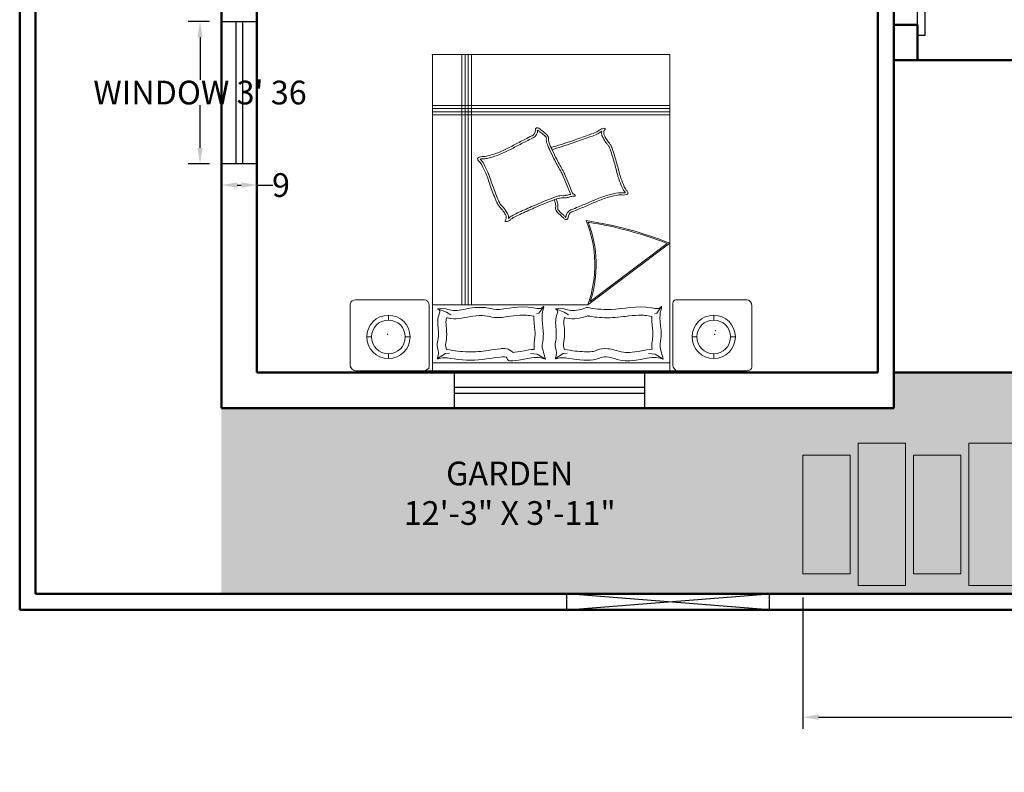
# Model space of a CAD drawing. Units: inches. Extents: x -466983 to 1020, y 324 to 318697.
# Tile 2 of 97: x 392 to 641, y 324 to 514. Entities that reach past the tile are written whole.
import ezdxf

# ---------------------------------------------------------------- set-up
doc = ezdxf.new("R2010")
doc.units = ezdxf.units.IN
doc.header["$MEASUREMENT"] = 0
for name, color, linetype, lineweight in [('A-ANNO-DIMS', 2, 'Continuous', 18), ('A-AREA-IDEN', 7, 'Continuous', 25), ('A-DOOR', 3, 'Continuous', 25), ('A-FLOR-PATT', 252, 'Continuous', 13), ('A-FURN', 8, 'Continuous', 18), ('A-GLAZ', 4, 'Continuous', 25), ('A-WALL', 7, 'Continuous', 50), ('L-SITE', 3, 'Continuous', 18)]:
    doc.layers.add(name, color=color, linetype=linetype, lineweight=lineweight)
doc.layers.add('K-Hatch', color=7, linetype='Continuous')
doc.styles.get("Standard").update_dxf_attribs({"font": 'arial.ttf'})
doc.dimstyles.get("Standard").update_dxf_attribs({"dimtxt": 6, "dimasz": 4, "dimexe": 3, "dimexo": 3, "dimgap": 0.09, "dimtad": 0, "dimtih": 1, "dimtoh": 1, "dimdec": 1, "dimzin": 0, "dimdsep": 46, "dimlunit": 3, "dimtxsty": 'Standard', "dimcen": 0.09, "dimadec": 0, "dimazin": 0, "dimtfac": 1, "dimtdec": 1, "dimtofl": 0, "dimtmove": 0, "dimatfit": 3, "dimfxl": 1, "dimtolj": 1, "dimtzin": 0, "dimarcsym": 0})

# ---------------------------------------------------------------- blocks, each defined once
blk = doc.blocks.new('Window 4 ft')
for p, q in [((1224.69, 893.77), (1233.69, 893.77)), ((1224.69, 845.77), (1224.69, 893.77)), ((1228.39, 845.77), (1228.39, 893.77)), ((1229.99, 893.77), (1229.99, 845.77)), ((1233.69, 893.77), (1233.69, 845.77)), ((1233.69, 845.77), (1224.69, 845.77))]:
    blk.add_line(p, q)
blk = doc.blocks.new("Window 3'")
for p, q in [((1346.92, 940.11), (1382.92, 940.11)), ((1346.92, 931.11), (1346.92, 940.11)), ((1382.92, 940.11), (1382.92, 931.11)), ((1346.92, 936.41), (1382.92, 936.41)), ((1382.92, 934.81), (1346.92, 934.81)), ((1382.92, 931.11), (1346.92, 931.11))]:
    blk.add_line(p, q)
blk = doc.blocks.new('Garden stone')
at = {"layer": 'K-Hatch'}
h = blk.add_hatch(color=256, dxfattribs=at)
h.dxf.hatch_style = 1
h.set_gradient(color1=(254, 234, 185), color2=(128, 128, 128), name='CYLINDER')
h.paths.add_polyline_path([(1828.21, 697.1), (1816.21, 697.1), (1816.21, 661.1), (1828.21, 661.1)])
h = blk.add_hatch(color=256, dxfattribs=at)
h.dxf.hatch_style = 1
h.set_gradient(color1=(254, 234, 185), color2=(128, 128, 128), name='CYLINDER')
h.paths.add_polyline_path([(1856.21, 697.1), (1844.21, 697.1), (1844.21, 661.1), (1856.21, 661.1)])
h = blk.add_hatch(color=256, dxfattribs=at)
h.dxf.hatch_style = 1
h.set_gradient(color1=(254, 234, 185), color2=(128, 128, 128), name='CYLINDER')
h.paths.add_polyline_path([(1884.21, 697.1), (1872.21, 697.1), (1872.21, 661.1), (1884.21, 661.1)])
h = blk.add_hatch(color=256, dxfattribs=at)
h.dxf.hatch_style = 1
h.set_gradient(color1=(254, 234, 185), color2=(128, 128, 128), name='CYLINDER')
h.paths.add_polyline_path([(1912.21, 697.1), (1900.21, 697.1), (1900.21, 661.1), (1912.21, 661.1)])
h = blk.add_hatch(color=256, dxfattribs=at)
h.dxf.hatch_style = 1
h.set_gradient(color1=(254, 234, 185), color2=(128, 128, 128), name='CYLINDER')
h.paths.add_polyline_path([(1940.21, 697.1), (1928.21, 697.1), (1928.21, 661.1), (1940.21, 661.1)])
h = blk.add_hatch(color=256, dxfattribs=at)
h.dxf.hatch_style = 1
h.set_gradient(color1=(254, 234, 185), color2=(128, 128, 128), name='CYLINDER')
h.paths.add_polyline_path([(1968.21, 697.1), (1956.21, 697.1), (1956.21, 661.1), (1968.21, 661.1)])
h = blk.add_hatch(color=256, dxfattribs=at)
h.dxf.hatch_style = 1
h.set_gradient(color1=(254, 234, 185), color2=(128, 128, 128), name='CYLINDER')
h.paths.add_polyline_path([(1996.21, 697.1), (1984.21, 697.1), (1984.21, 661.1), (1996.21, 661.1)])
h = blk.add_hatch(color=256, dxfattribs=at)
h.dxf.hatch_style = 1
h.set_gradient(color1=(254, 234, 185), color2=(128, 128, 128), name='CYLINDER')
h.paths.add_polyline_path([(2024.21, 697.1), (2012.21, 697.1), (2012.21, 661.1), (2024.21, 661.1)])
h = blk.add_hatch(color=256, dxfattribs=at)
h.dxf.hatch_style = 1
h.set_gradient(color1=(254, 234, 185), color2=(128, 128, 128), name='SPHERICAL')
h.paths.add_polyline_path([(1814.21, 694.1), (1802.21, 694.1), (1802.21, 664.1), (1814.21, 664.1)])
h = blk.add_hatch(color=256, dxfattribs=at)
h.dxf.hatch_style = 1
h.set_gradient(color1=(254, 234, 185), color2=(128, 128, 128), name='SPHERICAL')
h.paths.add_polyline_path([(1842.21, 694.1), (1830.21, 694.1), (1830.21, 664.1), (1842.21, 664.1)])
h = blk.add_hatch(color=256, dxfattribs=at)
h.dxf.hatch_style = 1
h.set_gradient(color1=(254, 234, 185), color2=(128, 128, 128), name='SPHERICAL')
h.paths.add_polyline_path([(1870.21, 694.1), (1858.21, 694.1), (1858.21, 664.1), (1870.21, 664.1)])
h = blk.add_hatch(color=256, dxfattribs=at)
h.dxf.hatch_style = 1
h.set_gradient(color1=(254, 234, 185), color2=(128, 128, 128), name='SPHERICAL')
h.paths.add_polyline_path([(1898.21, 694.1), (1886.21, 694.1), (1886.21, 664.1), (1898.21, 664.1)])
h = blk.add_hatch(color=256, dxfattribs=at)
h.dxf.hatch_style = 1
h.set_gradient(color1=(254, 234, 185), color2=(128, 128, 128), name='SPHERICAL')
h.paths.add_polyline_path([(1926.21, 694.1), (1914.21, 694.1), (1914.21, 664.1), (1926.21, 664.1)])
h = blk.add_hatch(color=256, dxfattribs=at)
h.dxf.hatch_style = 1
h.set_gradient(color1=(254, 234, 185), color2=(128, 128, 128), name='SPHERICAL')
h.paths.add_polyline_path([(1954.21, 694.1), (1942.21, 694.1), (1942.21, 664.1), (1954.21, 664.1)])
h = blk.add_hatch(color=256, dxfattribs=at)
h.dxf.hatch_style = 1
h.set_gradient(color1=(254, 234, 185), color2=(128, 128, 128), name='SPHERICAL')
h.paths.add_polyline_path([(1982.21, 694.1), (1970.21, 694.1), (1970.21, 664.1), (1982.21, 664.1)])
h = blk.add_hatch(color=256, dxfattribs=at)
h.dxf.hatch_style = 1
h.set_gradient(color1=(254, 234, 185), color2=(128, 128, 128), name='SPHERICAL')
h.paths.add_polyline_path([(2010.21, 694.1), (1998.21, 694.1), (1998.21, 664.1), (2010.21, 664.1)])
for points in [[(1816.21, 697.1), (1828.21, 697.1), (1828.21, 661.1), (1816.21, 661.1)], [(1844.21, 697.1), (1856.21, 697.1), (1856.21, 661.1), (1844.21, 661.1)], [(1872.21, 697.1), (1884.21, 697.1), (1884.21, 661.1), (1872.21, 661.1)], [(1900.21, 697.1), (1912.21, 697.1), (1912.21, 661.1), (1900.21, 661.1)], [(1928.21, 697.1), (1940.21, 697.1), (1940.21, 661.1), (1928.21, 661.1)], [(1956.21, 697.1), (1968.21, 697.1), (1968.21, 661.1), (1956.21, 661.1)], [(1984.21, 697.1), (1996.21, 697.1), (1996.21, 661.1), (1984.21, 661.1)], [(2012.21, 697.1), (2024.21, 697.1), (2024.21, 661.1), (2012.21, 661.1)], [(1802.21, 694.1), (1814.21, 694.1), (1814.21, 664.1), (1802.21, 664.1)], [(1830.21, 694.1), (1842.21, 694.1), (1842.21, 664.1), (1830.21, 664.1)], [(1858.21, 694.1), (1870.21, 694.1), (1870.21, 664.1), (1858.21, 664.1)], [(1886.21, 694.1), (1898.21, 694.1), (1898.21, 664.1), (1886.21, 664.1)], [(1914.21, 694.1), (1926.21, 694.1), (1926.21, 664.1), (1914.21, 664.1)], [(1942.21, 694.1), (1954.21, 694.1), (1954.21, 664.1), (1942.21, 664.1)], [(1970.21, 694.1), (1982.21, 694.1), (1982.21, 664.1), (1970.21, 664.1)], [(1998.21, 694.1), (2010.21, 694.1), (2010.21, 664.1), (1998.21, 664.1)]]:
    blk.add_lwpolyline(points, close=True)
blk = doc.blocks.new('A$C05F852CF')
for p, q in [((0, 3.0548), (0, 2.6659)), ((0.0306, 3.0783), (0.4692, 3.0783)), ((0.4692, 3.0783), (2.0768, 3.0783)), ((0.52, 3.0783), (0.52, 1.0783)), ((2.02, 3.0783), (2.02, 1.0783)), ((2.04, 3.05), (2.04, 2.6642)), ((2.0768, 3.0783), (2.5066, 3.0783)), ((0.2418, 2.9702), (0.2418, 3.0002)), ((0.5, 3.0423), (0.5, 2.6496)), ((0.52, 3.0283), (2.02, 3.0283)), ((0.5609, 3.0045), (0.5953, 2.9829)), ((0.5609, 3.0045), (0.6121, 2.9725)), ((1.2427, 2.9995), (1.1927, 2.9682)), ((2.2982, 2.9702), (2.2982, 3.0002)), ((2.54, 2.6547), (2.54, 3.0393)), ((0.6121, 2.9725), (0.6546, 2.9682)), ((1.1927, 2.9682), (1.1672, 2.9661)), ((0.1349, 2.8634), (0.1049, 2.8634)), ((0.3487, 2.8634), (0.3787, 2.8634)), ((2.1913, 2.8634), (2.1613, 2.8634)), ((2.4051, 2.8634), (2.4351, 2.8634)), ((0.2418, 2.7265), (0.2418, 2.7565)), ((2.2982, 2.7265), (2.2982, 2.7565)), ((0.5711, 2.6712), (0.6015, 2.7135)), ((0.6015, 2.7135), (0.6164, 2.7178)), ((1.1864, 2.7072), (1.1588, 2.7242)), ((1.2397, 2.6852), (1.1864, 2.7072)), ((0.0322, 2.6283), (0.4826, 2.6283)), ((1.0379, 2.6608), (0.52, 2.2697)), ((2.02, 2.6608), (1.0379, 2.6608)), ((1.7737, 2.6608), (1.7737, 1.0783)), ((1.7937, 2.6608), (1.7937, 1.0783)), ((1.8137, 2.6608), (1.8137, 1.0783)), ((1.8337, 2.6608), (1.8337, 1.0783)), ((2.0707, 2.6283), (2.5056, 2.6283)), ((0.52, 1.4597), (2.02, 1.4597)), ((0.52, 1.4397), (2.02, 1.4397)), ((0.52, 1.4197), (2.02, 1.4197)), ((0.52, 1.3997), (2.02, 1.3997)), ((0.52, 1.0783), (2.02, 1.0783)), ((0.726, 0.4346), (0.7377, 0.4444))]:
    blk.add_line(p, q)
for points in [[(1.3405, 2.9829), (1.306, 3.0045), (1.3573, 2.9725), (1.3998, 2.9682)], [(1.9879, 2.9995), (1.9379, 2.9682), (1.9124, 2.9661)], [(1.3162, 2.6712), (1.3467, 2.7135), (1.3616, 2.7178)], [(1.9848, 2.6852), (1.9315, 2.7072), (1.9039, 2.7242)]]:
    blk.add_lwpolyline(points)
for points in [[(1.0353, 2.1379, -0.173032), (1.022, 2.6388), (0.536, 2.2719, 0.053888)], [(1.7081, 1.7759, 0.101392), (1.7282, 1.7501, -0.223768), (1.7345, 1.736, -0.25558), (1.7315, 1.7308, -0.081563), (1.7151, 1.724, -0.071805), (1.6967, 1.7225, 0.069985), (1.6778, 1.7209, 0.03546), (1.6148, 1.7021, 0.029432), (1.5425, 1.6697, 0.001554), (1.5078, 1.6515, -0.00152), (1.4724, 1.6329, -0.004735), (1.4356, 1.6142, 0.00382), (1.3901, 1.5911, 0.296001), (1.3692, 1.5546, -0.649774), (1.3468, 1.5431, -0.02319), (1.3416, 1.5477, 0.0288), (1.3374, 1.5514, 0.005727), (1.3298, 1.557, -0.004358), (1.3198, 1.5645, -0.027528), (1.3001, 1.5812, -0.046214), (1.29, 1.5928, -0.194121), (1.2856, 1.6105, 0.133719), (1.2823, 1.6363, 0.011505), (1.2622, 1.682, 0.008882), (1.2338, 1.7401, 0.012426), (1.1937, 1.8139, -0.033612), (1.1801, 1.8418), (1.1552, 1.9026), (1.1361, 1.9495, 0.224341), (1.1204, 1.9638, -0.722772), (1.1202, 1.9734, -0.103513), (1.1242, 1.9739, 0.053465), (1.132, 1.9742, 0.030109), (1.1569, 1.9792, -0.031436), (1.1808, 1.984, -0.05324), (1.1971, 1.9844, 0.05518), (1.2128, 1.9849, 0.056271), (1.2402, 1.992, 0.0108), (1.3759, 2.0475, 0.00456), (1.4675, 2.0883, 0.01125), (1.5041, 2.106, 0.069394), (1.5235, 2.1196, -0.079756), (1.5405, 2.1311, -0.106399), (1.5562, 2.1345, -0.328642), (1.5608, 2.1312, -0.299547), (1.5587, 2.124, 0.189917), (1.5536, 2.1141, 0.033518), (1.5531, 2.1029, 0.075627), (1.554, 2.0981, 0.053489), (1.5579, 2.0898, 0.017838), (1.5727, 2.0672, 0.038394), (1.5932, 2.0425, -0.059529), (1.6058, 2.026, -0.035943), (1.6193, 1.9987, -0.011245), (1.6541, 1.9079, -0.006203), (1.6684, 1.8661, 0.010783), (1.6769, 1.8422, 0.019485), (1.6828, 1.8283, 0.005062)], [(1.6953, 1.7695, 0.098587), (1.7181, 1.7399, -0.040378), (1.7118, 1.7379, -0.071805), (1.6975, 1.7367, 0.069985), (1.6747, 1.7349, 0.03546), (1.6097, 1.7154, 0.029432), (1.5359, 1.6824, 0.001554), (1.5012, 1.6641, -0.00152), (1.4658, 1.6456, -0.004735), (1.4293, 1.627, 0.00382), (1.3835, 1.6038, 0.289814), (1.3549, 1.555, -0.018279), (1.3515, 1.5579, 0.0288), (1.3461, 1.5627, 0.005727), (1.3382, 1.5686, -0.004358), (1.3285, 1.5758, -0.027528), (1.31, 1.5916, -0.046214), (1.3016, 1.6012, -0.194121), (1.2997, 1.6085, 0.133719), (1.2955, 1.6417, 0.011505), (1.2752, 1.6881, 0.008882), (1.2465, 1.7466, 0.012426), (1.2061, 1.821, -0.033612), (1.1933, 1.8472), (1.1684, 1.908), (1.1493, 1.9549, 0.051417), (1.1455, 1.962, 0.017208), (1.1606, 1.9654, -0.031436), (1.1827, 1.9698, -0.05324), (1.196, 1.9702, 0.05518), (1.2149, 1.9708, 0.056271), (1.2453, 1.9787, 0.0108), (1.3816, 2.0344, 0.00456), (1.4734, 2.0753, 0.01125), (1.5106, 2.0933, 0.069394), (1.5332, 2.1091, -0.038161), (1.5392, 2.114, 0.029361), (1.5389, 2.1025, 0.075627), (1.5405, 2.0934, 0.053489), (1.5457, 2.0824, 0.017838), (1.5611, 2.0589, 0.038394), (1.583, 2.0326, -0.059529), (1.5935, 2.0187, -0.035943), (1.6061, 1.9933, -0.011245), (1.6406, 1.9031, -0.006203), (1.6549, 1.8617, 0.010783), (1.6635, 1.8371, 0.019485), (1.6699, 1.8222, 0.005062)]]:
    blk.add_lwpolyline(points, format="xyb", close=True)
for points in [[(1.27, 1.665, 0.025626), (1.2575, 1.662, 0.0108), (1.1179, 1.617, 0.00456), (1.0234, 1.5834, 0.01125), (0.9856, 1.5685, 0.069394), (0.9653, 1.5565, -0.079756), (0.9474, 1.5464, -0.106399), (0.9315, 1.5441, -0.328642), (0.9272, 1.5478, -0.299547), (0.9298, 1.5548, 0.189917), (0.9357, 1.5643, 0.033518), (0.9369, 1.5754, 0.075627), (0.9364, 1.5803, 0.053489), (0.9332, 1.5888, 0.017838), (0.9202, 1.6125, 0.038394), (0.9016, 1.6387, -0.059529), (0.8903, 1.6561, -0.035943), (0.8789, 1.6844, -0.011245), (0.8512, 1.7776, -0.006203), (0.8402, 1.8203, 0.010783), (0.8336, 1.8448, 0.019485), (0.8287, 1.8592, 0.005062), (0.8076, 1.9133, 0.101392), (0.7895, 1.9406, -0.223768), (0.7843, 1.9551, -0.25558), (0.7876, 1.9601, -0.081563), (0.8046, 1.9656, -0.071805), (0.823, 1.9657, 0.069985), (0.842, 1.9658, 0.03546), (0.9062, 1.9798, 0.029432), (0.9807, 2.0065, 0.001554), (1.0167, 2.022, -0.00152), (1.0535, 2.0378, -0.004735), (1.0916, 2.0536, 0.00382), (1.1388, 2.0731, 0.296001), (1.1624, 2.108, -0.649774), (1.1856, 2.1178, -0.02319), (1.1904, 2.1128, 0.0288), (1.1944, 2.1088, 0.005727), (1.2015, 2.1025, -0.004358), (1.2108, 2.0944, -0.027528), (1.2292, 2.0762, -0.046214), (1.2384, 2.0638, -0.194121), (1.2414, 2.0458, 0.133719), (1.2427, 2.0199, 0.005779), (1.2507, 1.9961)], [(1.2674, 1.6787, 0.025626), (1.2535, 1.6753, 0.0108), (1.1134, 1.6301, 0.00456), (1.0187, 1.5964, 0.01125), (0.9802, 1.5813, 0.069394), (0.9566, 1.5673, -0.042175), (0.9495, 1.5626, 0.031457), (0.9508, 1.5747, 0.075627), (0.9499, 1.5838, 0.053489), (0.9456, 1.595, 0.017838), (0.9321, 1.6196, 0.038394), (0.9123, 1.6476, -0.059529), (0.9028, 1.6622, -0.035943), (0.8922, 1.6886, -0.011245), (0.8646, 1.7812, -0.006203), (0.8536, 1.8236, 0.010783), (0.8469, 1.8487, 0.019485), (0.8417, 1.8641, 0.005062), (0.8204, 1.9185, 0.100237), (0.7996, 1.9501, -0.044209), (0.8066, 1.9519, -0.071805), (0.8211, 1.952, 0.069985), (0.8439, 1.9521, 0.03546), (0.9101, 1.9665, 0.029432), (0.9862, 1.9937, 0.001554), (1.0222, 2.0093, -0.00152), (1.0589, 2.025, -0.004735), (1.0968, 2.0408, 0.00382), (1.1442, 2.0604, 0.294287), (1.1763, 2.1074, -0.02184), (1.18, 2.1036, 0.0288), (1.1851, 2.0984, 0.005727), (1.1924, 2.092, -0.004358), (1.2016, 2.084, -0.027528), (1.2189, 2.0669, -0.046214), (1.2266, 2.0566, -0.194121), (1.2279, 2.0488, 0.133719), (1.2295, 2.0156, 0.005779), (1.2376, 1.9915, 0.005779)]]:
    blk.add_lwpolyline(points, format="xyb")
for centre, radius in [((0.2418, 2.8634), 0.1369), ((2.2982, 2.8634), 0.1369), ((0.2418, 2.8634), 0.1069), ((2.2982, 2.8634), 0.1069)]:
    blk.add_circle(centre, radius)
for centre, radius, start, end in [((1.7308, 2.407), 0.7379, 159.88462, 202.21936), ((1.4058, 4.5145), 2.4132, 248.46407, 261.46551)]:
    blk.add_arc(centre, radius, start, end)
for points in [[(0, 3.0548), (0, 3.0677), (0.0177, 3.0783), (0.0306, 3.0783)], [(0.5, 3.0423), (0.5, 3.0581), (0.485, 3.0783), (0.4692, 3.0783)], [(2.04, 3.05), (2.04, 3.0655), (2.0613, 3.0783), (2.0768, 3.0783)], [(2.5066, 3.0783), (2.5237, 3.0783), (2.54, 3.0564), (2.54, 3.0393)], [(0.0322, 2.6283), (0.0157, 2.6283), (0, 2.6494), (0, 2.6659)], [(0.5, 2.6496), (0.5, 2.6405), (0.4918, 2.6283), (0.4826, 2.6283)], [(2.04, 2.6642), (2.04, 2.6485), (2.055, 2.6283), (2.0707, 2.6283)], [(2.5056, 2.6283), (2.5201, 2.6283), (2.54, 2.6403), (2.54, 2.6547)]]:
    blk.add_open_spline(points, degree=3)
for points, knots in [([(0.5609, 3.0045), (0.565, 2.9818), (0.5836, 2.9366), (0.5776, 2.889), (0.5689, 2.8351), (0.5832, 2.7709), (0.5808, 2.7088), (0.5744, 2.6927), (0.5693, 2.6651), (0.5803, 2.6793), (0.5989, 2.6876), (0.7172, 2.6598), (0.8681, 2.7029), (1.0484, 2.6781), (1.0324, 2.6731), (1.1431, 2.7116), (1.202, 2.6757), (1.2459, 2.6867), (1.2222, 2.695), (1.2359, 2.7251), (1.2468, 2.781), (1.2288, 2.8492), (1.2515, 2.925), (1.2279, 2.9609), (1.2471, 3.0058), (1.2098, 2.9902), (1.1177, 3.0095), (0.956, 3.0159), (0.9532, 2.9758), (0.7999, 3.021), (0.7569, 3.0151), (0.5986, 2.9869), (0.561, 3.0049)], [16.816032, 16.816032, 16.816032, 16.816032, 79.038845, 88.513895, 147.565266, 227.196862, 259.685448, 283.955301, 296.511304, 302.432558, 320.230942, 354.322559, 575.279549, 734.72356, 845.740421, 943.033103, 1029.533967, 1032.845074, 1043.313584, 1065.311534, 1104.921835, 1208.53002, 1248.510714, 1303.102727, 1321.01326, 1329.647833, 1389.371624, 1571.817644, 1750.274161, 1823.189073, 1967.937033, 2020.912329, 2020.912329, 2020.912329, 2020.912329]), ([(1.306, 3.0045), (1.3102, 2.9818), (1.3287, 2.9366), (1.3228, 2.889), (1.314, 2.8351), (1.3284, 2.7709), (1.3259, 2.7088), (1.3196, 2.6927), (1.3144, 2.6651), (1.3254, 2.6793), (1.3441, 2.6876), (1.4624, 2.6598), (1.6132, 2.7029), (1.6436, 2.6781), (1.7775, 2.6731), (1.8882, 2.7116), (1.9472, 2.6757), (1.9911, 2.6867), (1.9673, 2.695), (1.981, 2.7251), (1.992, 2.781), (1.974, 2.8492), (1.9967, 2.925), (1.9731, 2.9609), (1.9922, 3.0058), (1.9549, 2.9902), (1.8628, 3.0095), (1.7011, 3.0159), (1.5483, 2.9758), (1.5451, 3.021), (1.5021, 3.0151), (1.3437, 2.9869), (1.3062, 3.0049)], [16.816032, 16.816032, 16.816032, 16.816032, 79.038845, 88.513895, 147.565266, 227.196862, 259.685448, 283.955301, 296.511304, 302.432558, 320.230942, 354.322559, 575.279549, 734.72356, 845.740421, 943.033103, 1029.533967, 1032.845074, 1043.313584, 1065.311534, 1104.921835, 1208.53002, 1248.510714, 1303.102727, 1321.01326, 1329.647833, 1389.371624, 1571.817644, 1750.274161, 1823.189073, 1967.937033, 2020.912329, 2020.912329, 2020.912329, 2020.912329]), ([(0.631, 2.9418), (0.6332, 2.9288), (0.633, 2.9104), (0.6308, 2.893), (0.6298, 2.8865), (0.628, 2.8726), (0.6273, 2.866), (0.6257, 2.8474), (0.6257, 2.8375), (0.629, 2.8013), (0.6345, 2.7696), (0.6337, 2.7333)], [67.285362, 67.285362, 67.285362, 67.285362, 87.399558, 87.399558, 107.513754, 107.513754, 127.62795, 127.62795, 167.856341, 167.856341, 238.127268, 238.127268, 238.127268, 238.127268]), ([(1.186, 2.943), (1.1557, 2.9456), (1.1387, 2.9502), (1.0976, 2.9551), (1.0776, 2.9567), (1.0342, 2.9582), (1.0123, 2.957), (0.991, 2.9533), (0.9902, 2.9517), (0.962, 2.9403), (0.9371, 2.935), (0.8851, 2.9413), (0.8522, 2.9513), (0.8033, 2.9629), (0.7938, 2.964), (0.755, 2.9608), (0.7319, 2.9572), (0.6794, 2.9481), (0.658, 2.9434), (0.631, 2.9418)], [1364.380335, 1364.380335, 1364.380335, 1364.380335, 1423.60231, 1423.60231, 1482.824284, 1482.824284, 1566.205036, 1566.205036, 1649.585789, 1649.585789, 1732.966542, 1732.966542, 1816.347295, 1816.347295, 1899.728048, 1899.728048, 1960.499853, 1960.499853, 1990.525565, 1990.525565, 1990.525565, 1990.525565]), ([(1.1845, 2.7412), (1.189, 2.7552), (1.1894, 2.765), (1.1874, 2.7998), (1.1843, 2.8219), (1.1844, 2.8664), (1.1882, 2.8901), (1.192, 2.9105), (1.1922, 2.9144), (1.1921, 2.9158), (1.1908, 2.9212), (1.1875, 2.9351), (1.1867, 2.9388), (1.186, 2.943)], [1072.516901, 1072.516901, 1072.516901, 1072.516901, 1129.100964, 1129.100964, 1185.685027, 1185.685027, 1226.035089, 1226.035089, 1249.281274, 1249.281274, 1272.52746, 1272.52746, 1279.689275, 1279.689275, 1279.689275, 1279.689275]), ([(1.3759, 2.942), (1.3781, 2.929), (1.378, 2.9106), (1.3757, 2.893), (1.3748, 2.8866), (1.373, 2.8727), (1.3722, 2.8661), (1.3706, 2.8475), (1.3707, 2.8375), (1.3739, 2.8012), (1.3795, 2.7694), (1.3787, 2.7331)], [67.156228, 67.156228, 67.156228, 67.156228, 87.297212, 87.297212, 107.438196, 107.438196, 127.57918, 127.57918, 167.861148, 167.861148, 238.25357, 238.25357, 238.25357, 238.25357]), ([(1.5104, 2.9621), (1.4964, 2.9606), (1.4732, 2.9568), (1.4226, 2.948), (1.4017, 2.9435), (1.3759, 2.942)], [1904.3965, 1904.3965, 1904.3965, 1904.3965, 1961.927876, 1961.927876, 1990.619445, 1990.619445, 1990.619445, 1990.619445]), ([(1.9314, 2.9432), (1.8997, 2.9459), (1.8822, 2.9507), (1.8387, 2.9557), (1.8168, 2.9572), (1.7515, 2.9587), (1.7088, 2.9551), (1.6403, 2.9447), (1.6154, 2.9402), (1.5795, 2.937), (1.5675, 2.9361), (1.5394, 2.9412), (1.5201, 2.9507), (1.5104, 2.9621)], [1364.265661, 1364.265661, 1364.265661, 1364.265661, 1426.240795, 1426.240795, 1488.215928, 1488.215928, 1612.166195, 1612.166195, 1689.92864, 1689.92864, 1733.064362, 1733.064362, 1768.978829, 1768.978829, 1768.978829, 1768.978829]), ([(1.9299, 2.7409), (1.9344, 2.755), (1.9348, 2.7648), (1.9328, 2.7996), (1.9297, 2.8217), (1.9298, 2.8662), (1.9336, 2.8899), (1.9374, 2.9105), (1.9376, 2.9144), (1.9375, 2.9159), (1.9362, 2.9214), (1.9329, 2.9353), (1.9321, 2.939), (1.9314, 2.9432)], [1072.238498, 1072.238498, 1072.238498, 1072.238498, 1128.864869, 1128.864869, 1185.491239, 1185.491239, 1225.989553, 1225.989553, 1249.326401, 1249.326401, 1272.66325, 1272.66325, 1279.788508, 1279.788508, 1279.788508, 1279.788508]), ([(0.6337, 2.7333), (0.6515, 2.7301), (0.6627, 2.7284), (0.6898, 2.7263), (0.7032, 2.726), (0.7436, 2.727), (0.7707, 2.73), (0.8409, 2.7383), (0.8881, 2.7432), (0.9755, 2.7406), (1.0125, 2.7357), (1.0356, 2.7309), (1.0369, 2.7307), (1.0381, 2.7304)], [345.4047, 345.4047, 345.4047, 345.4047, 383.386056, 383.386056, 421.367413, 421.367413, 497.330126, 497.330126, 611.561469, 611.561469, 725.792813, 725.792813, 732.434768, 732.434768, 732.434768, 732.434768]), ([(1.0381, 2.7304), (1.0497, 2.7345), (1.0742, 2.7435), (1.1251, 2.7504), (1.1528, 2.749), (1.1769, 2.7432), (1.1809, 2.7421), (1.1845, 2.7412)], [843.64503, 843.64503, 843.64503, 843.64503, 911.27572, 911.27572, 959.088062, 959.088062, 969.47998, 969.47998, 969.47998, 969.47998]), ([(1.3787, 2.7331), (1.3984, 2.7296), (1.4106, 2.7278), (1.4401, 2.7258), (1.4545, 2.7258), (1.4962, 2.7276), (1.5219, 2.7313), (1.5767, 2.7399), (1.6067, 2.7436), (1.6527, 2.7371), (1.662, 2.7326), (1.7084, 2.7282), (1.7364, 2.7276), (1.7849, 2.734), (1.8076, 2.7406), (1.8563, 2.7489), (1.8812, 2.7508), (1.914, 2.7451), (1.9226, 2.7428), (1.9299, 2.7409)], [345.267918, 345.267918, 345.267918, 345.267918, 387.167414, 387.167414, 429.06691, 429.06691, 512.865903, 512.865903, 629.317545, 629.317545, 745.769188, 745.769188, 834.622813, 834.622813, 901.414409, 901.414409, 948.921878, 948.921878, 969.679511, 969.679511, 969.679511, 969.679511])]:
    blk.add_open_spline(points, degree=3, knots=knots)
for p in [(0.2309, 2.8244), (0.2366, 2.8475), (2.3034, 2.8475), (2.02, 1.0783), (2.02, 1.0783)]:
    blk.add_point(p)
blk = doc.blocks.new('*U41')
for p, q in [((0, 0), (0, -6)), ((40, 0), (40, -6))]:
    blk.add_line(p, q)
blk.add_lwpolyline([(0, 0), (0, 40), (1.75, 40), (1.75, 0)], close=True)
blk.add_arc((0, 0), 40, 0, 90)
blk = doc.blocks.new('*D65')
at = {"layer": 'A-ANNO-DIMS', "color": 0, "lineweight": -2, "transparency": 16777216}
for p, q in [((439.81, 513.77), (434.41, 513.77)), ((437.41, 509.77), (437.41, 498.97)), ((437.41, 481.77), (437.41, 492.57)), ((439.81, 477.77), (434.41, 477.77))]:
    blk.add_line(p, q, dxfattribs=at)
at = {"layer": 'A-ANNO-DIMS', "color": 0, "transparency": 16777216}
for points in [[(436.74, 509.77), (438.07, 509.77), (437.41, 513.77)], [(436.74, 481.77), (438.07, 481.77), (437.41, 477.77)]]:
    blk.add_solid(points, dxfattribs=at)
at = {"layer": 'Defpoints', "color": 0, "transparency": 16777216}
for p in [(442.81, 513.77), (437.41, 477.77), (442.81, 477.77)]:
    blk.add_point(p, dxfattribs=at)
at = {"layer": 'A-ANNO-DIMS', "color": 0, "transparency": 16777216, "insert": (437.41, 495.77), "char_height": 6, "attachment_point": 5}
blk.add_mtext("\\A1;WINDOW 3' 36", dxfattribs=at)
blk = doc.blocks.new('*D66')
at = {"layer": 'A-ANNO-DIMS', "color": 0, "lineweight": -2, "transparency": 16777216}
for p, q in [((442.81, 474.77), (442.81, 469.37)), ((451.81, 474.77), (451.81, 469.37)), ((446.81, 472.37), (447.81, 472.37)), ((451.81, 472.37), (455.81, 472.37))]:
    blk.add_line(p, q, dxfattribs=at)
at = {"layer": 'A-ANNO-DIMS', "color": 0, "transparency": 16777216}
for points in [[(446.81, 473.04), (446.81, 471.7), (442.81, 472.37)], [(447.81, 473.04), (447.81, 471.7), (451.81, 472.37)]]:
    blk.add_solid(points, dxfattribs=at)
at = {"layer": 'Defpoints', "color": 0, "transparency": 16777216}
for p in [(442.81, 477.77), (451.81, 477.77), (451.81, 472.37)]:
    blk.add_point(p, dxfattribs=at)
at = {"layer": 'A-ANNO-DIMS', "color": 0, "transparency": 16777216, "insert": (457.87, 472.37), "char_height": 6, "attachment_point": 5}
blk.add_mtext('\\A1;9', dxfattribs=at)
blk = doc.blocks.new('*D115')
at = {"layer": 'A-ANNO-DIMS', "color": 0, "lineweight": -2, "transparency": 16777216}
for p, q in [((589.8, 368.07), (589.8, 334.77)), ((811.8, 368.07), (811.8, 334.77)), ((593.8, 337.77), (653.37, 337.77)), ((807.8, 337.77), (748.22, 337.77))]:
    blk.add_line(p, q, dxfattribs=at)
at = {"layer": 'A-ANNO-DIMS', "color": 0, "transparency": 16777216}
for points in [[(593.8, 338.44), (593.8, 337.1), (589.8, 337.77)], [(807.8, 338.44), (807.8, 337.1), (811.8, 337.77)]]:
    blk.add_solid(points, dxfattribs=at)
at = {"layer": 'Defpoints', "color": 0, "transparency": 16777216}
for p in [(589.8, 371.07), (811.8, 371.07), (811.8, 337.77)]:
    blk.add_point(p, dxfattribs=at)
at = {"layer": 'A-ANNO-DIMS', "color": 0, "transparency": 16777216, "insert": (700.8, 337.77), "char_height": 6, "attachment_point": 5}
blk.add_mtext('\\A1;STEPPING STONES 222', dxfattribs=at)

msp = doc.modelspace()

# ---------------------------------------------------------------- hatches: boundary and pattern name
at = {"layer": 'A-FLOR-PATT', "transparency": 33554661}
h = msp.add_hatch(color=256, dxfattribs=at)
h.dxf.hatch_style = 1
h.set_gradient(color1=(19, 155, 72), color2=(0, 107, 0), name='CYLINDER')
h.paths.add_polyline_path([(813.81, 503.94), (730.81, 503.94), (730.81, 424.94), (612.81, 424.94), (612.81, 415.94), (442.81, 415.94), (442.81, 368.94), (813.81, 368.94)])
h.paths.add_polyline_path([(771.8, 407.07), (783.8, 407.07), (783.8, 371.07), (771.8, 371.07)], flags=16)
h.paths.add_polyline_path([(755.8, 407.07), (755.8, 371.07), (743.8, 371.07), (743.8, 407.07)], flags=16)
h.paths.add_polyline_path([(769.8, 404.07), (769.8, 374.07), (757.8, 374.07), (757.8, 404.07)], flags=16)
h.paths.add_polyline_path([(785.8, 404.07), (797.8, 404.07), (797.8, 374.07), (785.8, 374.07)], flags=16)
h.paths.add_polyline_path([(741.8, 404.07), (741.8, 374.07), (729.8, 374.07), (729.8, 404.07)], flags=16)
h.paths.add_polyline_path([(799.8, 407.07), (811.8, 407.07), (811.8, 371.07), (799.8, 371.07)], flags=16)
h.paths.add_polyline_path([(727.8, 407.07), (727.8, 371.07), (715.8, 371.07), (715.8, 407.07)], flags=16)
h.paths.add_polyline_path([(713.8, 404.07), (713.8, 374.07), (701.8, 374.07), (701.8, 404.07)], flags=16)
h.paths.add_polyline_path([(699.8, 407.07), (699.8, 371.07), (687.8, 371.07), (687.8, 407.07)], flags=16)
h.paths.add_polyline_path([(685.8, 404.07), (685.8, 374.07), (673.8, 374.07), (673.8, 404.07)], flags=16)
h.paths.add_polyline_path([(671.8, 407.07), (671.8, 371.07), (659.8, 371.07), (659.8, 407.07)], flags=16)
h.paths.add_polyline_path([(657.8, 404.07), (657.8, 374.07), (645.8, 374.07), (645.8, 404.07)], flags=16)
h.paths.add_polyline_path([(643.8, 407.07), (643.8, 371.07), (631.8, 371.07), (631.8, 407.07)], flags=16)
h.paths.add_polyline_path([(629.8, 404.07), (629.8, 374.07), (617.8, 374.07), (617.8, 404.07)], flags=16)
h.paths.add_polyline_path([(615.8, 407.07), (615.8, 371.07), (603.8, 371.07), (603.8, 407.07)], flags=16)
h.paths.add_polyline_path([(601.8, 404.07), (601.8, 374.07), (589.8, 374.07), (589.8, 404.07)], flags=16)
at = {"layer": 'A-FLOR-PATT'}
h = msp.add_hatch(dxfattribs=at)
h.set_pattern_fill('GRASS', color=256, scale=6)
h.set_pattern_definition([(90, (-1212.4137, -290.035), (-4.242641, 4.242641), [1.125, -7.360281]), (45, (-1212.4137, -290.035), (-4.24264, 4.24264), [1.125, -4.875]), (135, (-1212.4137, -290.035), (-4.24264, -4.24264), [1.125, -4.875])])
h.paths.add_polyline_path([(813.81, 503.94), (730.81, 503.94), (730.81, 424.94), (612.81, 424.94), (612.81, 415.94), (442.81, 415.94), (442.81, 368.94), (813.81, 368.94)])
h.paths.add_polyline_path([(589.8, 404.07), (601.8, 404.07), (601.8, 374.07), (589.8, 374.07)], flags=16)
h.paths.add_polyline_path([(603.8, 407.07), (615.8, 407.07), (615.8, 371.07), (603.8, 371.07)], flags=16)
h.paths.add_polyline_path([(617.8, 404.07), (629.8, 404.07), (629.8, 374.07), (617.8, 374.07)], flags=16)
h.paths.add_polyline_path([(631.8, 407.07), (643.8, 407.07), (643.8, 371.07), (631.8, 371.07)], flags=16)
h.paths.add_polyline_path([(645.8, 404.07), (657.8, 404.07), (657.8, 374.07), (645.8, 374.07)], flags=16)
h.paths.add_polyline_path([(659.8, 407.07), (671.8, 407.07), (671.8, 371.07), (659.8, 371.07)], flags=16)
h.paths.add_polyline_path([(673.8, 404.07), (685.8, 404.07), (685.8, 374.07), (673.8, 374.07)], flags=16)
h.paths.add_polyline_path([(687.8, 407.07), (699.8, 407.07), (699.8, 371.07), (687.8, 371.07)], flags=16)
h.paths.add_polyline_path([(701.8, 404.07), (713.8, 404.07), (713.8, 374.07), (701.8, 374.07)], flags=16)
h.paths.add_polyline_path([(715.8, 407.07), (727.8, 407.07), (727.8, 371.07), (715.8, 371.07)], flags=16)
h.paths.add_polyline_path([(729.8, 404.07), (741.8, 404.07), (741.8, 374.07), (729.8, 374.07)], flags=16)
h.paths.add_polyline_path([(743.8, 407.07), (755.8, 407.07), (755.8, 371.07), (743.8, 371.07)], flags=16)
h.paths.add_polyline_path([(757.8, 404.07), (769.8, 404.07), (769.8, 374.07), (757.8, 374.07)], flags=16)
h.paths.add_polyline_path([(771.8, 407.07), (783.8, 407.07), (783.8, 371.07), (771.8, 371.07)], flags=16)
h.paths.add_polyline_path([(785.8, 404.07), (797.8, 404.07), (797.8, 374.07), (785.8, 374.07)], flags=16)
h.paths.add_polyline_path([(799.8, 407.07), (811.8, 407.07), (811.8, 371.07), (799.8, 371.07)], flags=16)

# ---------------------------------------------------------------- linework, layer by layer
at = {"layer": 'A-DOOR'}
for p, q in [((530.16, 364.94), (530.16, 368.94)), ((530.16, 364.94), (581.38, 368.94)), ((581.38, 364.94), (530.16, 368.94)), ((581.38, 364.94), (581.38, 368.94))]:
    msp.add_line(p, q, dxfattribs=at)
at = {"layer": 'A-WALL'}
for p, q in [((391.81, 364.94), (391.81, 1084.94)), ((442.81, 415.94), (442.81, 1084.94)), ((395.81, 368.94), (395.81, 1080.94)), ((612.81, 415.94), (612.81, 566.94)), ((451.81, 424.94), (451.81, 562.94)), ((608.81, 424.94), (608.81, 562.94)), ((618.81, 512.94), (612.81, 512.94)), ((618.81, 503.94), (618.81, 512.94)), ((618.81, 503.94), (612.81, 503.94)), ((813.81, 503.94), (618.81, 503.94)), ((608.81, 424.94), (451.81, 424.94)), ((608.81, 424.94), (451.81, 424.94)), ((730.81, 424.94), (612.81, 424.94)), ((612.81, 415.94), (442.81, 415.94)), ((987.81, 368.94), (395.81, 368.94)), ((991.81, 364.94), (391.81, 364.94))]:
    msp.add_line(p, q, dxfattribs=at)

# ---------------------------------------------------------------- block references
at = {"layer": 'A-DOOR', "xscale": 1.05, "yscale": 1.05, "zscale": 1.05}
msp.add_blockref('*U41', (618.81, 510.24), dxfattribs=at)
at = {"layer": 'A-FURN', "xscale": 40, "yscale": 40, "zscale": 40, "rotation": 180}
msp.add_blockref('A$C05F852CF', (576.97, 548.49), dxfattribs=at)
at = {"layer": 'A-GLAZ', "rotation": 270}
for name, p in [("Window 3'", (-488.3, 1860.69)), ('Window 4 ft', (-343.99, 1649.63))]:
    msp.add_blockref(name, p, dxfattribs=at)
at = {"layer": 'L-SITE'}
msp.add_blockref('Garden stone', (-1212.41, -290.04), dxfattribs=at)

# ---------------------------------------------------------------- texts
at = {"layer": 'A-AREA-IDEN', "insert": (400.94, 402.41), "char_height": 6, "attachment_point": 1}
msp.add_mtext_dynamic_manual_height_columns('\\pxqc;{\\fArial|b1|i0|c0|p34;GARDEN\\P12\'-3" X 3\'-11"}', width=229.5583, gutter_width=1, heights=[0], dxfattribs=at)

# ---------------------------------------------------------------- dimensions: what is measured, and where the dimension line sits
at = {"layer": 'A-ANNO-DIMS'}
dim = msp.add_linear_dim(base=(437.41, 477.77), p1=(442.81, 513.77), p2=(442.81, 477.77), angle=270, text="WINDOW 3' <>", dimstyle='Standard', override={"dimdec": 0, "dimlfac": 1, "dimrnd": 0, "dimzin": 0, "dimdsep": 46, "dimlunit": 2}, dxfattribs=at)
dim.commit()
dim.dimension.update_dxf_attribs({"geometry": '*D65', "text_midpoint": (437.41, 495.77)})
dim = msp.add_linear_dim(base=(451.81, 472.37), p1=(442.81, 477.77), p2=(451.81, 477.77), dimstyle='Standard', override={"dimdec": 0, "dimlfac": 1, "dimrnd": 0, "dimzin": 0, "dimdsep": 46, "dimlunit": 2}, dxfattribs=at)
dim.commit()
dim.dimension.update_dxf_attribs({"geometry": '*D66', "text_midpoint": (457.87, 472.37)})
dim = msp.add_linear_dim(base=(811.8, 337.77), p1=(589.8, 371.07), p2=(811.8, 371.07), text='STEPPING STONES <>', dimstyle='Standard', override={"dimdec": 0, "dimlfac": 1, "dimrnd": 0, "dimzin": 0, "dimdsep": 46, "dimlunit": 2}, dxfattribs=at)
dim.commit()
dim.dimension.update_dxf_attribs({"geometry": '*D115', "text_midpoint": (700.8, 337.77)})

doc.saveas('drawing.dxf')
